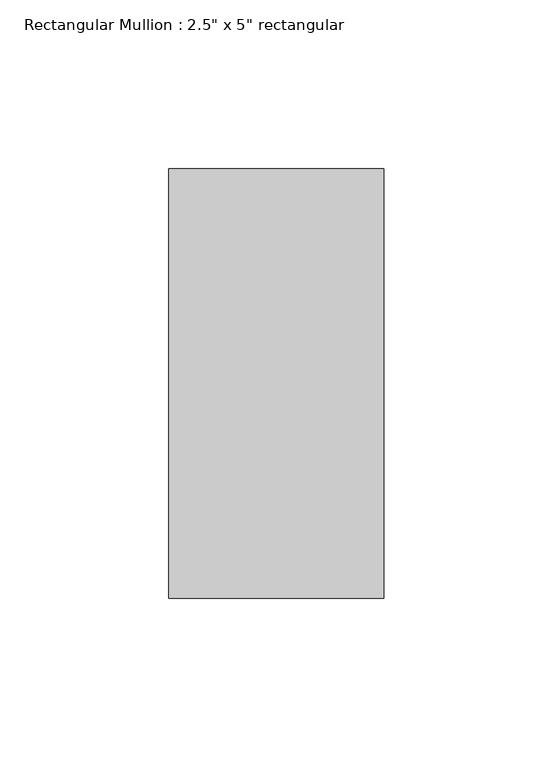
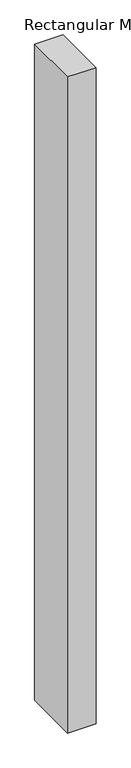
"""IFC4 building model written with IfcOpenShell, lengths in millimetres: member geometry."""

from ifc_helpers import new_model, si_unit, frame, origin, place, context, project, spatial, polyline, outline, extrude, source, transform, mapped, element, save


def member_fff16b5b(model_context):
    return source(origin(), model_context, "Body", "SweptSolid", [
        extrude(outline(polyline([(31.75, 63.5), (31.75, -63.5), (-31.75, -63.5), (-31.75, 63.5), (31.75, 63.5)])), frame((0.0, 0.0, -1547.2824814), z_axis=(0.0, 0.0, 1.0), x_axis=(1.0, 0.0, 0.0)), (0.0, 0.0, 1.0), 1547.2824814),
    ])


if __name__ == "__main__":
    model = new_model("IFC4")
    model_context = context("Model", 3, world=origin())
    ifc_project = project(units=[si_unit("LENGTHUNIT", "METRE", prefix="MILLI")], contexts=[model_context])
    site = spatial("IfcSite", under=ifc_project)
    building = spatial("IfcBuilding", under=site)
    placement = place(None, origin())
    member_shape = member_fff16b5b(model_context)
    element("IfcMember", 1, ObjectType="Rectangular Mullion : 2.5\" x 5\" rectangular", at=placement, inside=building, context=model_context, shape_type="MappedRepresentation", body=[
        mapped(member_shape, transform((0.0, 0.0, 0.0), x_axis=(1.0, 0.0, 0.0), y_axis=(0.0, 1.0, 0.0), z_axis=(0.0, 0.0, 1.0))),
    ])
    save(model, "model.ifc")

# Revit data of these elements
# Type "Rectangular Mullion : 2.5\" x 5\" rectangular"
#   built-in parameter 1007304 = 0.416667 (stored number, unit not read)
#   built-in parameter 1007301 = 0.104167 (stored number, unit not read)
#   built-in parameter 1007300 = 0.104167 (stored number, unit not read)
# Element 1 (IfcMember, "Rectangular Mullion : 2.5\" x 5\" rectangular")
#   Materials on its faces: "Aluminum"
# Materials
#   "Aluminum": class "Metal", colour RGB 247 247 247, transparency 0, Description = "Aluminum 6061", Cost = 0
